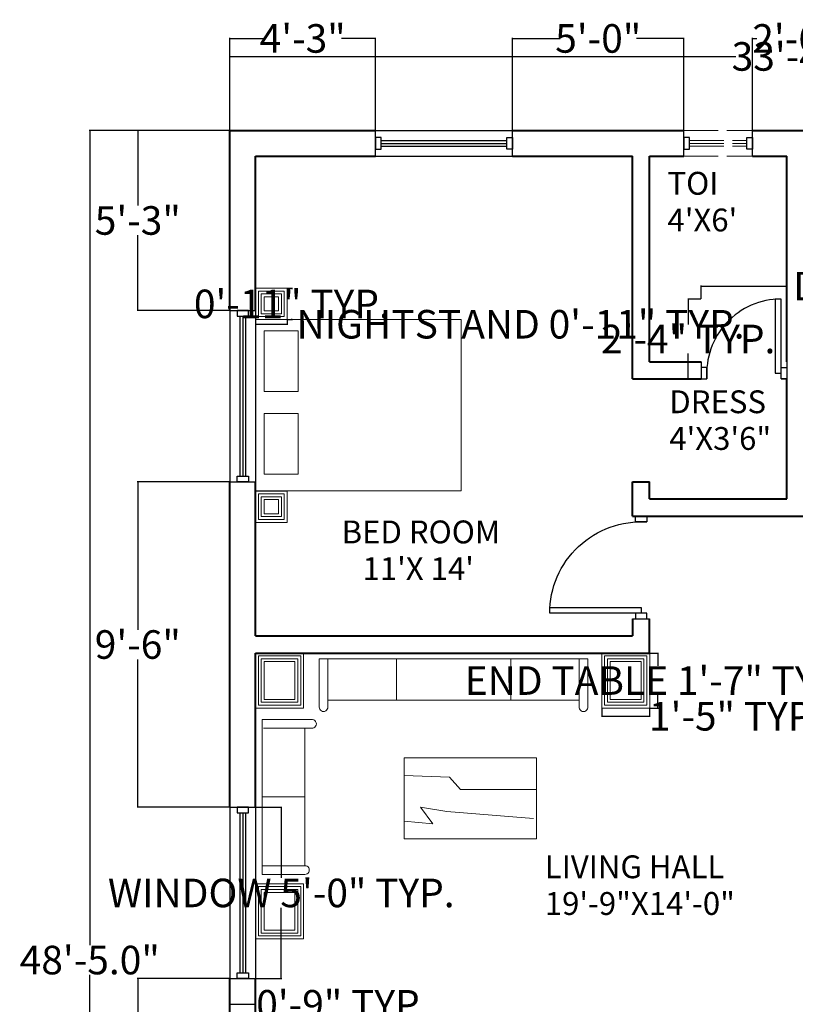
# Model space of a CAD drawing. Units: inches. Extents: x -413 to 212, y 1694 to 2633.
# Tile 4 of 5: x -413 to -141, y 2279 to 2624. Entities that reach past the tile are written whole.
import ezdxf

# ---------------------------------------------------------------- set-up
doc = ezdxf.new("R2010")
doc.units = ezdxf.units.IN
doc.header["$MEASUREMENT"] = 0
doc.linetypes.add('ACAD_ISO02W100', pattern=[15, 12, -3])
for name, color, linetype, lineweight in [('A-ANNO-DIMS', 5, 'Continuous', 18), ('A-AREA-IDEN', 251, 'Continuous', 25), ('A-GLAZ-OVHD', 2, 'ACAD_ISO02W100', 18), ('A-GLAZ-VENT', 2, 'Continuous', 25), ('door', 4, 'Continuous', 25), ('furniture', 1, 'Continuous', 18), ('wall', 20, 'Continuous', 40), ('window', 6, 'Continuous', 25)]:
    doc.layers.add(name, color=color, linetype=linetype, lineweight=lineweight)
doc.styles.get("Standard").update_dxf_attribs({"font": 'arial.ttf'})
doc.dimstyles.get("Standard").update_dxf_attribs({"dimtxt": 10, "dimasz": 0.18, "dimexe": 0.18, "dimexo": 0.0625, "dimgap": 0.09, "dimtad": 0, "dimtih": 1, "dimtoh": 1, "dimdec": 1, "dimzin": 0, "dimdsep": 46, "dimlunit": 3, "dimtxsty": 'Standard', "dimblk": 'ARCHTICK', "dimcen": 0.09, "dimadec": 0, "dimazin": 0, "dimtfac": 1, "dimtdec": 1, "dimtofl": 0, "dimtmove": 0, "dimatfit": 3, "dimfxl": 1, "dimtolj": 1, "dimtzin": 0, "dimarcsym": 0})

# ---------------------------------------------------------------- blocks, each defined once
blk = doc.blocks.new('_ArchTick')
at = {"color": 0, "linetype": 'ByBlock', "const_width": 0.15}
blk.add_lwpolyline([(-0.5, -0.5), (0.5, 0.5)], dxfattribs=at)
blk = doc.blocks.new('*D2')
at = {"layer": 'A-ANNO-DIMS', "color": 0, "lineweight": -2, "transparency": 16777216}
for p, q in [((-339.04, 2585.48), (-388.23, 2585.48)), ((-388.05, 2585.48), (-388.05, 2300.18)), ((-388.05, 2004.48), (-388.05, 2289.79)), ((-339.04, 2004.48), (-388.23, 2004.48))]:
    blk.add_line(p, q, dxfattribs=at)
at = {"layer": 'Defpoints', "color": 0, "transparency": 16777216}
for p in [(-388.05, 2585.48), (-338.98, 2585.48), (-338.98, 2004.48)]:
    blk.add_point(p, dxfattribs=at)
at = {"layer": 'A-ANNO-DIMS', "color": 0, "lineweight": -2, "transparency": 16777216, "xscale": 0.18, "yscale": 0.18, "zscale": 0.18}
for p, rotation in [((-388.05, 2585.48), 90), ((-388.05, 2004.48), 270)]:
    blk.add_blockref('_ArchTick', p, dxfattribs=dict(at, rotation=rotation))
at = {"layer": 'A-ANNO-DIMS', "color": 0, "transparency": 16777216, "insert": (-388.05, 2294.98), "char_height": 10, "attachment_point": 5}
blk.add_mtext('\\A1;48\'-5.0"', dxfattribs=at)
blk = doc.blocks.new('*D3')
at = {"layer": 'A-ANNO-DIMS', "color": 0, "lineweight": -2, "transparency": 16777216}
for p, q in [((-338.98, 2585.55), (-338.98, 2611.61)), ((-338.98, 2611.43), (-161.81, 2611.43)), ((61.52, 2611.43), (-115.64, 2611.43)), ((61.52, 2585.55), (61.52, 2611.61))]:
    blk.add_line(p, q, dxfattribs=at)
at = {"layer": 'Defpoints', "color": 0, "transparency": 16777216}
for p in [(61.52, 2611.43), (-338.98, 2585.48), (61.52, 2585.48)]:
    blk.add_point(p, dxfattribs=at)
at = {"layer": 'A-ANNO-DIMS', "color": 0, "lineweight": -2, "transparency": 16777216, "xscale": 0.18, "yscale": 0.18, "zscale": 0.18, "rotation": 180}
blk.add_blockref('_ArchTick', (-338.98, 2611.43), dxfattribs=at)
at = {"layer": 'A-ANNO-DIMS', "color": 0, "lineweight": -2, "transparency": 16777216, "xscale": 0.18, "yscale": 0.18, "zscale": 0.18}
blk.add_blockref('_ArchTick', (61.52, 2611.43), dxfattribs=at)
at = {"layer": 'A-ANNO-DIMS', "color": 0, "transparency": 16777216, "insert": (-138.73, 2611.43), "char_height": 10, "attachment_point": 5}
blk.add_mtext('\\A1;33\'-4.5"', dxfattribs=at)
blk = doc.blocks.new('WINDOW-48IN')
for p, q in [((0, 0), (0, 9)), ((0, 9), (48, 9)), ((48, 0), (48, 9)), ((2, 5.5), (46, 5.5)), ((2, 4.5), (46, 4.5)), ((2, 3.5), (46, 3.5)), ((0, 0), (48, 0))]:
    blk.add_line(p, q)
for points in [[(0, 2.5), (2, 2.5), (2, 6.5), (0, 6.5)], [(48, 2.5), (46, 2.5), (46, 6.5), (48, 6.5)]]:
    blk.add_lwpolyline(points, close=True)
blk = doc.blocks.new('WINDOW-60IN')
for p, q in [((0, 60), (9, 60)), ((0, 60), (0, 0)), ((9, 60), (9, 0)), ((3.5, 58), (3.5, 2)), ((4.5, 58), (4.5, 2)), ((5.5, 58), (5.5, 2)), ((0, 0), (9, 0))]:
    blk.add_line(p, q)
for points in [[(2.5, 60), (2.5, 58), (6.5, 58), (6.5, 60)], [(2.5, 0), (2.5, 2), (6.5, 2), (6.5, 0)]]:
    blk.add_lwpolyline(points, close=True)
blk = doc.blocks.new('VENT-JAMBS-24IN')
for p, q in [((0, 0), (0, 9)), ((24, 0), (24, 9))]:
    blk.add_line(p, q)
for points in [[(0, 2.5), (2, 2.5), (2, 6.5), (0, 6.5)], [(24, 2.5), (22, 2.5), (22, 6.5), (24, 6.5)]]:
    blk.add_lwpolyline(points, close=True)
blk = doc.blocks.new('VENT-PANEL-24IN')
for p, q in [((0, 9), (24, 9)), ((2, 5.5), (22, 5.5)), ((2, 4.5), (22, 4.5)), ((2, 3.5), (22, 3.5)), ((0, 0), (24, 0))]:
    blk.add_line(p, q)
blk = doc.blocks.new('DOOR-SWING-36IN')
for p, q in [((3, 34), (-3, 34)), ((3, -2), (-3, -2))]:
    blk.add_line(p, q)
for points in [[(-2, 34), (-2, 32), (2, 32), (2, 34)], [(-2, -2), (-2, 0), (2, 0), (2, -2)], [(0, 0), (32, 0), (32, 2), (0, 2)]]:
    blk.add_lwpolyline(points, close=True)
blk.add_arc((0, 0), 32, 0, 93.5833)
blk = doc.blocks.new('DOOR-SWING-30IN')
for points in [[(0, 0), (0, 26), (-2, 26), (-2, 0)], [(-28, -2), (-26, -2), (-26, 2), (-28, 2)], [(2, -2), (0, -2), (0, 2), (2, 2)]]:
    blk.add_lwpolyline(points, close=True)
blk.add_arc((0, 0), 26, 90, 184.4117)
blk = doc.blocks.new('BED-DOUBLE-60X72')
for p, q in [((0, 60), (72, 60)), ((72, 0), (72, 60)), ((0, 0), (72, 0))]:
    blk.add_line(p, q)
for points in [[(3.06, 34.82), (14.86, 34.82), (14.86, 56.09), (3.06, 56.09)], [(3.06, 5.88), (14.86, 5.88), (14.86, 27.14), (3.06, 27.14)]]:
    blk.add_lwpolyline(points, close=True)
blk = doc.blocks.new('NIGHTSTAND-STEPPED')
for points in [[(0, 0), (11.05, 0), (11.05, 10.95), (0, 10.95)], [(0, 0), (11.05, 0), (11.05, 10.95), (0, 10.95)], [(1, 1), (10.05, 1), (10.05, 9.95), (1, 9.95)], [(2, 2), (9.05, 2), (9.05, 8.95), (2, 8.95)], [(3, 3), (8.05, 3), (8.05, 7.95), (3, 7.95)]]:
    blk.add_lwpolyline(points, close=True)
blk = doc.blocks.new('SOFA-THREE-SEAT')
for points in [[(0, 1.47), (0, 18.46), (94.05, 18.46), (94.05, 1.28)], [(3, 1.47), (3, 18.46)], [(27, 4), (27, 18.46)], [(67.05, 18.46), (67.05, 4)], [(91.05, 18.46), (91.05, 1.28)], [(91.05, 4), (3, 4)]]:
    blk.add_lwpolyline(points)
for centre, radius, start, end in [((1.5, 1.51), 1.5, 178.5982, 1.4018), ((92.55, 1.52), 1.52, 171.0874, 8.9126)]:
    blk.add_arc(centre, radius, start, end)
blk = doc.blocks.new('SOFA-TWO-SEAT')
for points in [[(0, 0), (0, 54.18), (17.18, 54.18)], [(0.47, 51.18), (17.65, 51.18)], [(14.93, 51.18), (14.93, 3.18)], [(0, 27.18), (14.93, 27.18)], [(15.01, 3), (0, 3)], [(0, 0), (14.93, 0)]]:
    blk.add_lwpolyline(points)
for centre, radius, start, end in [((17.41, 52.68), 1.52, 261.0874, 98.9126), ((14.97, 1.5), 1.5, 268.5982, 91.4018)]:
    blk.add_arc(centre, radius, start, end)
blk = doc.blocks.new('TABLE-COFFEE')
for p, q in [((0, 22.18), (0, 22.18)), ((0, 22.18), (15.93, 21.7)), ((15.93, 21.7), (19.8, 17.36)), ((19.8, 17.36), (46.35, 17.36)), ((10.14, 5.3), (5.79, 11.09)), ((5.79, 11.09), (14.97, 9.64)), ((14.97, 9.64), (45.38, 7.23)), ((0, 6.27), (0, 6.27)), ((0, 6.27), (10.14, 5.3))]:
    blk.add_line(p, q)
blk.add_lwpolyline([(0, 28.45), (46.35, 28.45), (46.35, 0), (0, 0)], close=True)
blk = doc.blocks.new('TABLE-END')
for points in [[(0, 19.24), (16.8, 19.24), (16.8, 0), (0, 0)], [(1, 18.24), (15.8, 18.24), (15.8, 1), (1, 1)], [(2, 17.24), (14.8, 17.24), (14.8, 2), (2, 2)], [(3, 16.24), (13.8, 16.24), (13.8, 3), (3, 3)]]:
    blk.add_lwpolyline(points, close=True)
blk = doc.blocks.new('*D29')
at = {"layer": 'A-ANNO-DIMS', "color": 0, "lineweight": -2, "transparency": 16777216}
for p, q in [((-329.91, 2348.48), (-320.8, 2348.48)), ((-320.98, 2348.48), (-320.98, 2323.75)), ((-320.98, 2288.48), (-320.98, 2313.22)), ((-329.91, 2288.48), (-320.8, 2288.48))]:
    blk.add_line(p, q, dxfattribs=at)
at = {"layer": 'Defpoints', "color": 0, "transparency": 16777216}
for p in [(-329.98, 2348.48), (-320.98, 2348.48), (-329.98, 2288.48)]:
    blk.add_point(p, dxfattribs=at)
at = {"layer": 'A-ANNO-DIMS', "color": 0, "lineweight": -2, "transparency": 16777216, "xscale": 0.18, "yscale": 0.18, "zscale": 0.18}
for p, rotation in [((-320.98, 2348.48), 90), ((-320.98, 2288.48), 270)]:
    blk.add_blockref('_ArchTick', p, dxfattribs=dict(at, rotation=rotation))
at = {"layer": 'A-ANNO-DIMS', "color": 0, "transparency": 16777216, "insert": (-320.98, 2318.48), "char_height": 10, "attachment_point": 5}
blk.add_mtext('\\A1;WINDOW 5\'-0" TYP.', dxfattribs=at)
blk = doc.blocks.new('*D30')
at = {"layer": 'A-ANNO-DIMS', "color": 0, "lineweight": -2, "transparency": 16777216}
for p, q in [((-338.98, 2288.42), (-338.98, 2279.3)), ((-329.98, 2288.42), (-329.98, 2279.3)), ((-338.98, 2279.48), (-329.98, 2279.48)), ((-329.98, 2279.48), (-329.8, 2279.48))]:
    blk.add_line(p, q, dxfattribs=at)
at = {"layer": 'Defpoints', "color": 0, "transparency": 16777216}
for p in [(-338.98, 2288.48), (-329.98, 2288.48), (-329.98, 2279.48)]:
    blk.add_point(p, dxfattribs=at)
at = {"layer": 'A-ANNO-DIMS', "color": 0, "lineweight": -2, "transparency": 16777216, "xscale": 0.18, "yscale": 0.18, "zscale": 0.18, "rotation": 180}
blk.add_blockref('_ArchTick', (-338.98, 2279.48), dxfattribs=at)
at = {"layer": 'A-ANNO-DIMS', "color": 0, "lineweight": -2, "transparency": 16777216, "xscale": 0.18, "yscale": 0.18, "zscale": 0.18}
blk.add_blockref('_ArchTick', (-329.98, 2279.48), dxfattribs=at)
at = {"layer": 'A-ANNO-DIMS', "color": 0, "transparency": 16777216, "insert": (-299.23, 2279.48), "char_height": 10, "attachment_point": 5}
blk.add_mtext('\\A1;0\'-9" TYP.', dxfattribs=at)
blk = doc.blocks.new('*D33')
at = {"layer": 'A-ANNO-DIMS', "color": 0, "lineweight": -2, "transparency": 16777216}
for p, q in [((-191.91, 2402.48), (-188.91, 2402.48)), ((-189.09, 2402.48), (-189.09, 2397.98)), ((-189.09, 2383.24), (-189.09, 2387.75)), ((-191.91, 2383.24), (-188.91, 2383.24))]:
    blk.add_line(p, q, dxfattribs=at)
at = {"layer": 'Defpoints', "color": 0, "transparency": 16777216}
for p in [(-191.98, 2402.48), (-189.09, 2402.48), (-191.98, 2383.24)]:
    blk.add_point(p, dxfattribs=at)
at = {"layer": 'A-ANNO-DIMS', "color": 0, "lineweight": -2, "transparency": 16777216, "xscale": 0.18, "yscale": 0.18, "zscale": 0.18}
for p, rotation in [((-189.09, 2402.48), 90), ((-189.09, 2383.24), 270)]:
    blk.add_blockref('_ArchTick', p, dxfattribs=dict(at, rotation=rotation))
at = {"layer": 'A-ANNO-DIMS', "color": 0, "transparency": 16777216, "insert": (-189.09, 2392.86), "char_height": 10, "attachment_point": 5}
blk.add_mtext('\\A1;END TABLE 1\'-7" TYP.', dxfattribs=at)
blk = doc.blocks.new('*D34')
at = {"layer": 'A-ANNO-DIMS', "color": 0, "lineweight": -2, "transparency": 16777216}
for p, q in [((-208.77, 2383.18), (-208.77, 2380.17)), ((-191.98, 2383.18), (-191.98, 2380.17)), ((-208.77, 2380.35), (-191.98, 2380.35)), ((-191.98, 2380.35), (-191.8, 2380.35))]:
    blk.add_line(p, q, dxfattribs=at)
at = {"layer": 'Defpoints', "color": 0, "transparency": 16777216}
for p in [(-208.77, 2383.24), (-191.98, 2383.24), (-191.98, 2380.35)]:
    blk.add_point(p, dxfattribs=at)
at = {"layer": 'A-ANNO-DIMS', "color": 0, "lineweight": -2, "transparency": 16777216, "xscale": 0.18, "yscale": 0.18, "zscale": 0.18, "rotation": 180}
blk.add_blockref('_ArchTick', (-208.77, 2380.35), dxfattribs=at)
at = {"layer": 'A-ANNO-DIMS', "color": 0, "lineweight": -2, "transparency": 16777216, "xscale": 0.18, "yscale": 0.18, "zscale": 0.18}
blk.add_blockref('_ArchTick', (-191.98, 2380.35), dxfattribs=at)
at = {"layer": 'A-ANNO-DIMS', "color": 0, "transparency": 16777216, "insert": (-161.7, 2380.35), "char_height": 10, "attachment_point": 5}
blk.add_mtext('\\A1;1\'-5" TYP.', dxfattribs=at)
blk = doc.blocks.new('*D35')
at = {"layer": 'A-ANNO-DIMS', "color": 0, "lineweight": -2, "transparency": 16777216}
for p, q in [((-173.98, 2526.55), (-173.98, 2531.16)), ((-173.98, 2530.98), (-143.98, 2530.98)), ((-143.98, 2526.55), (-143.98, 2531.16)), ((-143.98, 2530.98), (-143.8, 2530.98))]:
    blk.add_line(p, q, dxfattribs=at)
at = {"layer": 'Defpoints', "color": 0, "transparency": 16777216}
for p in [(-143.98, 2530.98), (-173.98, 2526.48), (-143.98, 2526.48)]:
    blk.add_point(p, dxfattribs=at)
at = {"layer": 'A-ANNO-DIMS', "color": 0, "lineweight": -2, "transparency": 16777216, "xscale": 0.18, "yscale": 0.18, "zscale": 0.18, "rotation": 180}
blk.add_blockref('_ArchTick', (-173.98, 2530.98), dxfattribs=at)
at = {"layer": 'A-ANNO-DIMS', "color": 0, "lineweight": -2, "transparency": 16777216, "xscale": 0.18, "yscale": 0.18, "zscale": 0.18}
blk.add_blockref('_ArchTick', (-143.98, 2530.98), dxfattribs=at)
at = {"layer": 'A-ANNO-DIMS', "color": 0, "transparency": 16777216, "insert": (-90.58, 2530.98), "char_height": 10, "attachment_point": 5}
blk.add_mtext('\\A1;DOOR 2\'-6" TYP.', dxfattribs=at)
blk = doc.blocks.new('*D36')
at = {"layer": 'A-ANNO-DIMS', "color": 0, "lineweight": -2, "transparency": 16777216}
for p, q in [((-174.04, 2526.48), (-178.66, 2526.48)), ((-178.48, 2526.48), (-178.48, 2517.6)), ((-178.48, 2498.48), (-178.48, 2507.37)), ((-174.04, 2498.48), (-178.66, 2498.48))]:
    blk.add_line(p, q, dxfattribs=at)
at = {"layer": 'Defpoints', "color": 0, "transparency": 16777216}
for p in [(-178.48, 2526.48), (-173.98, 2526.48), (-173.98, 2498.48)]:
    blk.add_point(p, dxfattribs=at)
at = {"layer": 'A-ANNO-DIMS', "color": 0, "lineweight": -2, "transparency": 16777216, "xscale": 0.18, "yscale": 0.18, "zscale": 0.18}
for p, rotation in [((-178.48, 2526.48), 90), ((-178.48, 2498.48), 270)]:
    blk.add_blockref('_ArchTick', p, dxfattribs=dict(at, rotation=rotation))
at = {"layer": 'A-ANNO-DIMS', "color": 0, "transparency": 16777216, "insert": (-178.48, 2512.48), "char_height": 10, "attachment_point": 5}
blk.add_mtext('\\A1;2\'-4" TYP.', dxfattribs=at)
blk = doc.blocks.new('*D43')
at = {"layer": 'A-ANNO-DIMS', "color": 0, "lineweight": -2, "transparency": 16777216}
for p, q in [((-329.98, 2519.24), (-329.98, 2517.46)), ((-329.98, 2517.64), (-318.93, 2517.64)), ((-318.93, 2519.24), (-318.93, 2517.46)), ((-318.93, 2517.64), (-318.75, 2517.64))]:
    blk.add_line(p, q, dxfattribs=at)
at = {"layer": 'Defpoints', "color": 0, "transparency": 16777216}
for p in [(-329.98, 2519.3), (-318.93, 2519.3), (-318.93, 2517.64)]:
    blk.add_point(p, dxfattribs=at)
at = {"layer": 'A-ANNO-DIMS', "color": 0, "lineweight": -2, "transparency": 16777216, "xscale": 0.18, "yscale": 0.18, "zscale": 0.18, "rotation": 180}
blk.add_blockref('_ArchTick', (-329.98, 2517.64), dxfattribs=at)
at = {"layer": 'A-ANNO-DIMS', "color": 0, "lineweight": -2, "transparency": 16777216, "xscale": 0.18, "yscale": 0.18, "zscale": 0.18}
blk.add_blockref('_ArchTick', (-318.93, 2517.64), dxfattribs=at)
at = {"layer": 'A-ANNO-DIMS', "color": 0, "transparency": 16777216, "insert": (-237.19, 2517.64), "char_height": 10, "attachment_point": 5}
blk.add_mtext('\\A1;NIGHTSTAND 0\'-11" TYP.', dxfattribs=at)
blk = doc.blocks.new('*D44')
at = {"layer": 'A-ANNO-DIMS', "color": 0, "lineweight": -2, "transparency": 16777216}
for p, q in [((-318.87, 2530.25), (-317.09, 2530.25)), ((-317.27, 2530.25), (-317.27, 2529.97)), ((-318.87, 2519.3), (-317.09, 2519.3)), ((-317.27, 2519.3), (-317.27, 2519.58))]:
    blk.add_line(p, q, dxfattribs=at)
at = {"layer": 'Defpoints', "color": 0, "transparency": 16777216}
for p in [(-318.93, 2530.25), (-317.27, 2530.25), (-318.93, 2519.3)]:
    blk.add_point(p, dxfattribs=at)
at = {"layer": 'A-ANNO-DIMS', "color": 0, "lineweight": -2, "transparency": 16777216, "xscale": 0.18, "yscale": 0.18, "zscale": 0.18}
for p, rotation in [((-317.27, 2530.25), 90), ((-317.27, 2519.3), 270)]:
    blk.add_blockref('_ArchTick', p, dxfattribs=dict(at, rotation=rotation))
at = {"layer": 'A-ANNO-DIMS', "color": 0, "transparency": 16777216, "insert": (-317.27, 2524.77), "char_height": 10, "attachment_point": 5}
blk.add_mtext('\\A1;0\'-11" TYP.', dxfattribs=at)
blk = doc.blocks.new('*D64')
at = {"layer": 'A-ANNO-DIMS', "color": 0, "lineweight": -2, "transparency": 16777216}
for p, q in [((-338.98, 2585.55), (-338.98, 2617.91)), ((-338.98, 2617.73), (-327.06, 2617.73)), ((-287.98, 2617.73), (-299.89, 2617.73)), ((-287.98, 2585.55), (-287.98, 2617.91))]:
    blk.add_line(p, q, dxfattribs=at)
at = {"layer": 'Defpoints', "color": 0, "transparency": 16777216}
for p in [(-287.98, 2617.73), (-338.98, 2585.48), (-287.98, 2585.48)]:
    blk.add_point(p, dxfattribs=at)
at = {"layer": 'A-ANNO-DIMS', "color": 0, "lineweight": -2, "transparency": 16777216, "xscale": 0.18, "yscale": 0.18, "zscale": 0.18, "rotation": 180}
blk.add_blockref('_ArchTick', (-338.98, 2617.73), dxfattribs=at)
at = {"layer": 'A-ANNO-DIMS', "color": 0, "lineweight": -2, "transparency": 16777216, "xscale": 0.18, "yscale": 0.18, "zscale": 0.18}
blk.add_blockref('_ArchTick', (-287.98, 2617.73), dxfattribs=at)
at = {"layer": 'A-ANNO-DIMS', "color": 0, "transparency": 16777216, "insert": (-313.48, 2617.73), "char_height": 10, "attachment_point": 5}
blk.add_mtext('\\A1;4\'-3"', dxfattribs=at)
blk = doc.blocks.new('*D65')
at = {"layer": 'A-ANNO-DIMS', "color": 0, "lineweight": -2, "transparency": 16777216}
for p, q in [((-239.98, 2585.55), (-239.98, 2617.91)), ((-239.98, 2617.73), (-223.36, 2617.73)), ((-179.98, 2617.73), (-196.59, 2617.73)), ((-179.98, 2585.55), (-179.98, 2617.91))]:
    blk.add_line(p, q, dxfattribs=at)
at = {"layer": 'Defpoints', "color": 0, "transparency": 16777216}
for p in [(-179.98, 2617.73), (-239.98, 2585.48), (-179.98, 2585.48)]:
    blk.add_point(p, dxfattribs=at)
at = {"layer": 'A-ANNO-DIMS', "color": 0, "lineweight": -2, "transparency": 16777216, "xscale": 0.18, "yscale": 0.18, "zscale": 0.18, "rotation": 180}
blk.add_blockref('_ArchTick', (-239.98, 2617.73), dxfattribs=at)
at = {"layer": 'A-ANNO-DIMS', "color": 0, "lineweight": -2, "transparency": 16777216, "xscale": 0.18, "yscale": 0.18, "zscale": 0.18}
blk.add_blockref('_ArchTick', (-179.98, 2617.73), dxfattribs=at)
at = {"layer": 'A-ANNO-DIMS', "color": 0, "transparency": 16777216, "insert": (-209.98, 2617.73), "char_height": 10, "attachment_point": 5}
blk.add_mtext('\\A1;5\'-0"', dxfattribs=at)
blk = doc.blocks.new('*D66')
at = {"layer": 'A-ANNO-DIMS', "color": 0, "lineweight": -2, "transparency": 16777216}
for p, q in [((-155.98, 2585.55), (-155.98, 2617.91)), ((-155.98, 2617.73), (-154.44, 2617.73)), ((-125.98, 2617.73), (-127.51, 2617.73)), ((-125.98, 2585.55), (-125.98, 2617.91))]:
    blk.add_line(p, q, dxfattribs=at)
at = {"layer": 'Defpoints', "color": 0, "transparency": 16777216}
for p in [(-125.98, 2617.73), (-155.98, 2585.48), (-125.98, 2585.48)]:
    blk.add_point(p, dxfattribs=at)
at = {"layer": 'A-ANNO-DIMS', "color": 0, "lineweight": -2, "transparency": 16777216, "xscale": 0.18, "yscale": 0.18, "zscale": 0.18, "rotation": 180}
blk.add_blockref('_ArchTick', (-155.98, 2617.73), dxfattribs=at)
at = {"layer": 'A-ANNO-DIMS', "color": 0, "lineweight": -2, "transparency": 16777216, "xscale": 0.18, "yscale": 0.18, "zscale": 0.18}
blk.add_blockref('_ArchTick', (-125.98, 2617.73), dxfattribs=at)
at = {"layer": 'A-ANNO-DIMS', "color": 0, "transparency": 16777216, "insert": (-140.98, 2617.73), "char_height": 10, "attachment_point": 5}
blk.add_mtext('\\A1;2\'-6"', dxfattribs=at)
blk = doc.blocks.new('*D68')
at = {"layer": 'A-ANNO-DIMS', "color": 0, "lineweight": -2, "transparency": 16777216}
for p, q in [((-339.04, 2585.48), (-371.41, 2585.48)), ((-371.23, 2585.48), (-371.23, 2559.18)), ((-371.23, 2522.48), (-371.23, 2548.79)), ((-339.04, 2522.48), (-371.41, 2522.48))]:
    blk.add_line(p, q, dxfattribs=at)
at = {"layer": 'Defpoints', "color": 0, "transparency": 16777216}
for p in [(-338.98, 2585.48), (-371.23, 2522.48), (-338.98, 2522.48)]:
    blk.add_point(p, dxfattribs=at)
at = {"layer": 'A-ANNO-DIMS', "color": 0, "lineweight": -2, "transparency": 16777216, "xscale": 0.18, "yscale": 0.18, "zscale": 0.18}
for p, rotation in [((-371.23, 2585.48), 90), ((-371.23, 2522.48), 270)]:
    blk.add_blockref('_ArchTick', p, dxfattribs=dict(at, rotation=rotation))
at = {"layer": 'A-ANNO-DIMS', "color": 0, "transparency": 16777216, "insert": (-371.23, 2553.98), "char_height": 10, "attachment_point": 5}
blk.add_mtext('\\A1;5\'-3"', dxfattribs=at)
blk = doc.blocks.new('*D69')
at = {"layer": 'A-ANNO-DIMS', "color": 0, "lineweight": -2, "transparency": 16777216}
for p, q in [((-339.04, 2462.48), (-371.41, 2462.48)), ((-371.23, 2462.48), (-371.23, 2410.68)), ((-371.23, 2348.48), (-371.23, 2400.29)), ((-339.04, 2348.48), (-371.41, 2348.48))]:
    blk.add_line(p, q, dxfattribs=at)
at = {"layer": 'Defpoints', "color": 0, "transparency": 16777216}
for p in [(-338.98, 2462.48), (-371.23, 2348.48), (-338.98, 2348.48)]:
    blk.add_point(p, dxfattribs=at)
at = {"layer": 'A-ANNO-DIMS', "color": 0, "lineweight": -2, "transparency": 16777216, "xscale": 0.18, "yscale": 0.18, "zscale": 0.18}
for p, rotation in [((-371.23, 2462.48), 90), ((-371.23, 2348.48), 270)]:
    blk.add_blockref('_ArchTick', p, dxfattribs=dict(at, rotation=rotation))
at = {"layer": 'A-ANNO-DIMS', "color": 0, "transparency": 16777216, "insert": (-371.23, 2405.48), "char_height": 10, "attachment_point": 5}
blk.add_mtext('\\A1;9\'-6"', dxfattribs=at)
blk = doc.blocks.new('*D70')
at = {"layer": 'A-ANNO-DIMS', "color": 0, "lineweight": -2, "transparency": 16777216}
for p, q in [((-339.04, 2288.48), (-371.41, 2288.48)), ((-371.23, 2288.48), (-371.23, 2242.68)), ((-371.23, 2186.48), (-371.23, 2232.29)), ((-339.04, 2186.48), (-371.41, 2186.48))]:
    blk.add_line(p, q, dxfattribs=at)
at = {"layer": 'Defpoints', "color": 0, "transparency": 16777216}
for p in [(-338.98, 2288.48), (-371.23, 2186.48), (-338.98, 2186.48)]:
    blk.add_point(p, dxfattribs=at)
at = {"layer": 'A-ANNO-DIMS', "color": 0, "lineweight": -2, "transparency": 16777216, "xscale": 0.18, "yscale": 0.18, "zscale": 0.18}
for p, rotation in [((-371.23, 2288.48), 90), ((-371.23, 2186.48), 270)]:
    blk.add_blockref('_ArchTick', p, dxfattribs=dict(at, rotation=rotation))
at = {"layer": 'A-ANNO-DIMS', "color": 0, "transparency": 16777216, "insert": (-371.23, 2237.48), "char_height": 10, "attachment_point": 5}
blk.add_mtext('\\A1;8\'-6"', dxfattribs=at)

msp = doc.modelspace()

# ---------------------------------------------------------------- linework, layer by layer
at = {"layer": 'door'}
for p, q in [((-173.98, 2504.48), (-173.98, 2498.48)), ((-143.98, 2504.48), (-143.98, 2498.48)), ((-173.98, 2498.48), (-171.9, 2498.48)), ((-145.98, 2498.48), (-143.98, 2498.48))]:
    msp.add_line(p, q, dxfattribs=at)
at = {"layer": 'wall'}
for p, q in [((-338.98, 2585.48), (-287.98, 2585.48)), ((-338.98, 2522.48), (-338.98, 2585.48)), ((-239.98, 2585.48), (-179.98, 2585.48)), ((-155.98, 2585.48), (-125.98, 2585.48)), ((-329.98, 2576.48), (-287.98, 2576.48)), ((-329.98, 2522.48), (-329.98, 2576.48)), ((-239.98, 2576.48), (-197.98, 2576.48)), ((-197.98, 2498.48), (-197.98, 2576.48)), ((-191.98, 2504.48), (-191.98, 2576.48)), ((-191.98, 2576.48), (-179.98, 2576.48)), ((-155.98, 2576.48), (-143.98, 2576.48)), ((-143.98, 2504.48), (-143.98, 2576.48)), ((-191.98, 2504.48), (-173.98, 2504.48)), ((-197.98, 2498.48), (-173.98, 2498.48)), ((-143.98, 2456.48), (-143.98, 2498.48)), ((-338.98, 2348.48), (-338.98, 2462.48)), ((-329.98, 2408.48), (-329.98, 2462.48)), ((-197.98, 2450.48), (-197.98, 2462.48)), ((-197.98, 2462.48), (-191.98, 2462.48)), ((-191.98, 2456.48), (-191.98, 2462.48)), ((-191.98, 2456.48), (-143.98, 2456.48)), ((-197.98, 2450.48), (-83.98, 2450.48)), ((-197.98, 2414.48), (-197.98, 2408.48)), ((-191.98, 2402.48), (-191.98, 2414.48)), ((-329.98, 2408.48), (-197.98, 2408.48)), ((-329.98, 2402.48), (-191.98, 2402.48)), ((-329.98, 2348.48), (-329.98, 2402.48)), ((-338.98, 2186.48), (-338.98, 2288.48)), ((-329.98, 2234.48), (-329.98, 2288.48))]:
    msp.add_line(p, q, dxfattribs=at)

# ---------------------------------------------------------------- block references
at = {"layer": 'A-GLAZ-OVHD'}
msp.add_blockref('VENT-PANEL-24IN', (-179.98, 2576.49), dxfattribs=at)
at = {"layer": 'A-GLAZ-VENT'}
msp.add_blockref('VENT-JAMBS-24IN', (-179.98, 2576.49), dxfattribs=at)
at = {"layer": 'door'}
msp.add_blockref('DOOR-SWING-30IN', (-145.98, 2500.48), dxfattribs=at)
at = {"layer": 'door', "extrusion": (0, 0, -1), "zscale": -1}
msp.add_blockref('DOOR-SWING-36IN', (194.98, 2416.48), dxfattribs=at)
at = {"layer": 'furniture'}
for name, p in [('NIGHTSTAND-STEPPED', (-329.98, 2519.3)), ('BED-DOUBLE-60X72', (-329.98, 2459.3)), ('NIGHTSTAND-STEPPED', (-329.98, 2448.26)), ('TABLE-END', (-329.98, 2383.24)), ('SOFA-THREE-SEAT', (-307.68, 2382.02)), ('TABLE-END', (-208.77, 2383.24)), ('SOFA-TWO-SEAT', (-327.63, 2325)), ('TABLE-COFFEE', (-278, 2337.38)), ('TABLE-END', (-329.98, 2302.45))]:
    msp.add_blockref(name, p, dxfattribs=at)
at = {"layer": 'window'}
for name, p in [('WINDOW-48IN', (-287.98, 2576.49)), ('WINDOW-60IN', (-338.98, 2462.49)), ('WINDOW-60IN', (-338.98, 2288.49))]:
    msp.add_blockref(name, p, dxfattribs=at)

# ---------------------------------------------------------------- texts
at = {"layer": 'A-AREA-IDEN'}
for s, p in [('TOI', (-185.74, 2563)), ("4'X6'", (-185.74, 2550.15)), ('DRESS ', (-185.1, 2486.49)), ('4\'X3\'6"', (-185.1, 2473.64)), ('BED ROOM ', (-299.86, 2440.91)), ("   11'X 14'", (-299.86, 2428.06)), ('LIVING HALL', (-228.71, 2323.64)), ('19\'-9"X14\'-0"', (-228.71, 2310.79))]:
    msp.add_text(s, height=8, dxfattribs=at).set_placement(p)

# ---------------------------------------------------------------- dimensions: what is measured, and where the dimension line sits
at = {"layer": 'A-ANNO-DIMS'}
for base, p1, p2, override, picture, middle in [((-287.98, 2617.73), (-338.98, 2585.48), (-287.98, 2585.48), {"dimdec": 1, "dimlfac": 1, "dimrnd": 0, "dimzin": 1, "dimdsep": 46, "dimlunit": 4, "dimfrac": 2}, '*D64', (-313.48, 2617.73)), ((-179.98, 2617.73), (-239.98, 2585.48), (-179.98, 2585.48), {"dimdec": 1, "dimlfac": 1, "dimrnd": 0, "dimzin": 1, "dimdsep": 46, "dimlunit": 4, "dimfrac": 2}, '*D65', (-209.98, 2617.73)), ((-125.98, 2617.73), (-155.98, 2585.48), (-125.98, 2585.48), {"dimdec": 1, "dimlfac": 1, "dimrnd": 0, "dimzin": 1, "dimdsep": 46, "dimlunit": 4, "dimfrac": 2}, '*D66', (-140.98, 2617.73)), ((61.52, 2611.43), (-338.98, 2585.48), (61.52, 2585.48), {"dimclrd": 0, "dimclre": 0, "dimclrt": 0}, '*D3', (-138.73, 2611.43))]:
    dim = msp.add_linear_dim(base=base, p1=p1, p2=p2, dimstyle='Standard', override=override, dxfattribs=at)
    dim.commit()
    dim.dimension.update_dxf_attribs({"geometry": picture, "text_midpoint": middle})
for base, p1, p2, override, picture, middle in [((-388.05, 2585.48), (-338.98, 2004.48), (-338.98, 2585.48), {"dimclrd": 0, "dimclre": 0, "dimclrt": 0}, '*D2', (-388.05, 2294.98)), ((-371.23, 2522.48), (-338.98, 2585.48), (-338.98, 2522.48), {"dimdec": 1, "dimlfac": 1, "dimrnd": 0, "dimzin": 1, "dimdsep": 46, "dimlunit": 4, "dimfrac": 2}, '*D68', (-371.23, 2553.98)), ((-371.23, 2348.48), (-338.98, 2462.48), (-338.98, 2348.48), {"dimdec": 1, "dimlfac": 1, "dimrnd": 0, "dimzin": 1, "dimdsep": 46, "dimlunit": 4, "dimfrac": 2}, '*D69', (-371.23, 2405.48)), ((-371.23, 2186.48), (-338.98, 2288.48), (-338.98, 2186.48), {"dimdec": 1, "dimlfac": 1, "dimrnd": 0, "dimzin": 1, "dimdsep": 46, "dimlunit": 4, "dimfrac": 2}, '*D70', (-371.23, 2237.48))]:
    dim = msp.add_linear_dim(base=base, p1=p1, p2=p2, angle=90, dimstyle='Standard', override=override, dxfattribs=at)
    dim.commit()
    dim.dimension.update_dxf_attribs({"geometry": picture, "text_midpoint": middle})
for base, p1, p2, text, picture, middle in [((-143.98, 2530.98), (-173.98, 2526.48), (-143.98, 2526.48), 'DOOR <> TYP.', '*D35', (-90.58, 2530.98)), ((-318.928, 2517.6429), (-329.9757, 2519.3), (-318.928, 2519.3), 'NIGHTSTAND <> TYP.', '*D43', (-237.1949, 2517.6429)), ((-191.98, 2380.35), (-208.77, 2383.24), (-191.98, 2383.24), '<> TYP.', '*D34', (-161.7, 2380.35)), ((-329.98, 2279.48), (-338.98, 2288.48), (-329.98, 2288.48), '<> TYP.', '*D30', (-299.23, 2279.48))]:
    dim = msp.add_linear_dim(base=base, p1=p1, p2=p2, text=text, dimstyle='Standard', override={"dimdec": 1, "dimlfac": 1, "dimrnd": 0, "dimzin": 1, "dimdsep": 46, "dimlunit": 4, "dimfrac": 2}, dxfattribs=at)
    dim.commit()
    dim.dimension.update_dxf_attribs({"geometry": picture, "text_midpoint": middle})
for base, p1, p2, text, picture, middle in [((-317.2709, 2530.248), (-318.928, 2519.3), (-318.928, 2530.248), '<> TYP.', '*D44', (-317.2709, 2524.774)), ((-178.48, 2526.48), (-173.98, 2498.48), (-173.98, 2526.48), '<> TYP.', '*D36', (-178.48, 2512.48)), ((-189.09, 2402.48), (-191.98, 2383.24), (-191.98, 2402.48), 'END TABLE <> TYP.', '*D33', (-189.09, 2392.86)), ((-320.98, 2348.48), (-329.98, 2288.48), (-329.98, 2348.48), 'WINDOW <> TYP.', '*D29', (-320.98, 2318.48))]:
    dim = msp.add_linear_dim(base=base, p1=p1, p2=p2, angle=90, text=text, dimstyle='Standard', override={"dimdec": 1, "dimlfac": 1, "dimrnd": 0, "dimzin": 1, "dimdsep": 46, "dimlunit": 4, "dimfrac": 2}, dxfattribs=at)
    dim.commit()
    dim.dimension.update_dxf_attribs({"geometry": picture, "text_midpoint": middle})

doc.saveas('drawing.dxf')
